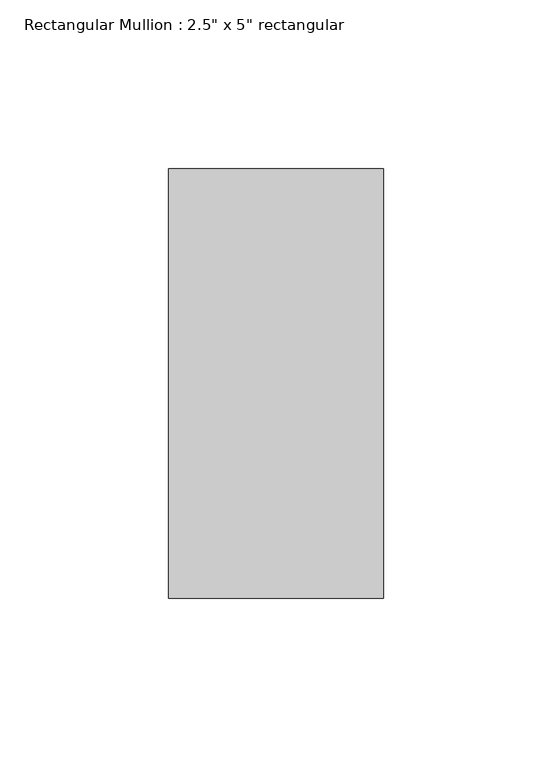
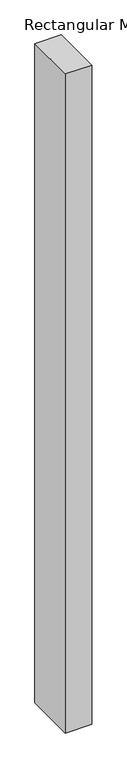
"""IFC4 building model written with IfcOpenShell, lengths in millimetres: member geometry."""

from ifc_helpers import new_model, si_unit, frame, origin, place, context, project, spatial, polyline, outline, extrude, source, transform, mapped, element, save


def member_8c071503(model_context):
    return source(origin(), model_context, "Body", "SweptSolid", [
        extrude(outline(polyline([(31.75, 63.5), (31.75, -63.5), (-31.75, -63.5), (-31.75, 63.5), (31.75, 63.5)])), frame((0.0, 0.0, -1681.1349385), z_axis=(0.0, 0.0, 1.0), x_axis=(1.0, 0.0, 0.0)), (0.0, 0.0, 1.0), 1681.1349385),
    ])


if __name__ == "__main__":
    model = new_model("IFC4")
    model_context = context("Model", 3, world=origin())
    ifc_project = project(units=[si_unit("LENGTHUNIT", "METRE", prefix="MILLI")], contexts=[model_context])
    site = spatial("IfcSite", under=ifc_project)
    building = spatial("IfcBuilding", under=site)
    placement = place(None, origin())
    member_shape = member_8c071503(model_context)
    element("IfcMember", 1, ObjectType="Rectangular Mullion : 2.5\" x 5\" rectangular", at=placement, inside=building, context=model_context, shape_type="MappedRepresentation", body=[
        mapped(member_shape, transform((0.0, 0.0, 0.0), x_axis=(1.0, 0.0, 0.0), y_axis=(0.0, 1.0, 0.0), z_axis=(0.0, 0.0, 1.0))),
    ])
    save(model, "model.ifc")

# Revit data of these elements
# Type "Rectangular Mullion : 2.5\" x 5\" rectangular"
#   built-in parameter 1007304 = 0.416667 (stored number, unit not read)
#   built-in parameter 1007301 = 0.104167 (stored number, unit not read)
#   built-in parameter 1007300 = 0.104167 (stored number, unit not read)
# Element 1 (IfcMember, "Rectangular Mullion : 2.5\" x 5\" rectangular")
#   Materials on its faces: "Aluminum"
# Materials
#   "Aluminum": class "Metal", colour RGB 247 247 247, transparency 0, Description = "Aluminum 6061", Cost = 0
